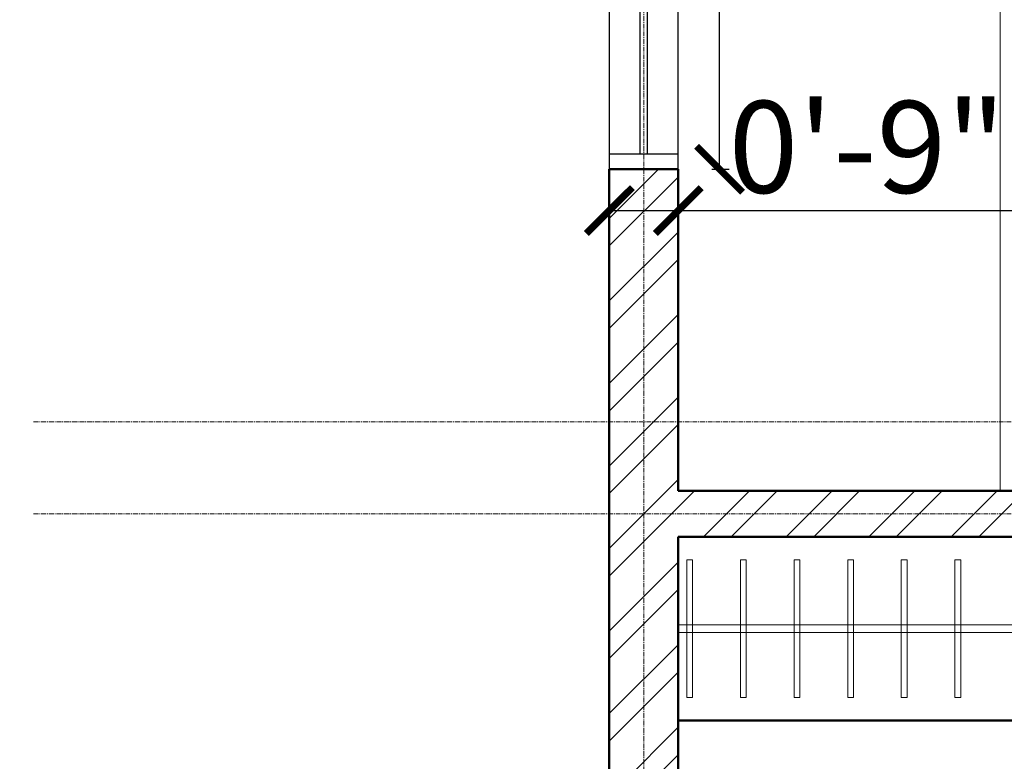
# Model space of a CAD drawing. Units: inches. Extents: x 261 to 2725, y 291 to 1454.
# Tile 19 of 35: x 1166 to 1295, y 644 to 741. Entities that reach past the tile are written whole.
import ezdxf

# ---------------------------------------------------------------- set-up
doc = ezdxf.new("R2010")
doc.units = ezdxf.units.IN
doc.linetypes.add('CENTER', pattern=[2, 1.25, -0.25, 0.25, -0.25])
for name, color, linetype, lineweight in [('A-ANNO-DIMS', 136, 'Continuous', 18), ('A-FLOR-FIXT', 145, 'Continuous', 18), ('A-FURN', 30, 'Continuous', 18), ('A-GLAZ', 150, 'Continuous', 25), ('A-GRID', 251, 'CENTER', 13), ('A-WALL', 222, 'Continuous', 50), ('A-WALL-PATT', 243, 'Continuous', 13)]:
    doc.layers.add(name, color=color, linetype=linetype, lineweight=lineweight)
doc.styles.get("Standard").update_dxf_attribs({"font": 'arial.ttf'})
doc.dimstyles.new('ISO-25', dxfattribs={"dimtxt": 12, "dimasz": 6, "dimexe": 1.25, "dimexo": 0.625, "dimtad": 1, "dimdec": 0, "dimlunit": 3, "dimtxsty": 'Standard', "dimblk": 'ARCHTICK', "dimcen": 2.5, "dimadec": 0, "dimazin": 0, "dimtfac": 1, "dimtdec": 0, "dimtmove": 0, "dimatfit": 3, "dimfxl": 1, "dimfxlon": 1, "dimarcsym": 0})

# ---------------------------------------------------------------- blocks, each defined once
blk = doc.blocks.new('WIN-36')
for p, q in [((1252.08, 755.47), (1243.08, 755.47)), ((1247.08, 755.47), (1247.08, 723.47)), ((1248.08, 723.47), (1248.08, 755.47)), ((1243.08, 723.47), (1252.08, 723.47))]:
    blk.add_line(p, q)
blk.add_lwpolyline([(1252.08, 721.47), (1252.08, 757.47), (1243.08, 757.47), (1243.08, 721.47)], close=True)
blk = doc.blocks.new('_ArchTick')
at = {"color": 0, "linetype": 'ByBlock', "const_width": 0.15}
blk.add_lwpolyline([(-0.5, -0.5), (0.5, 0.5)], dxfattribs=at)
blk = doc.blocks.new('*D59')
at = {"layer": 'A-ANNO-DIMS', "color": 0, "lineweight": -2, "ltscale": 0.07, "transparency": 16777216}
for p, q in [((1257.48, 757.47), (1257.48, 946.37)), ((1256.48, 757.47), (1258.73, 757.47)), ((1257.48, 721.47), (1257.48, 757.47)), ((1256.48, 721.47), (1258.73, 721.47))]:
    blk.add_line(p, q, dxfattribs=at)
at = {"layer": 'Defpoints', "color": 0, "ltscale": 0.07, "transparency": 16777216}
for p in [(1252.08, 757.47), (1257.48, 757.47), (1252.08, 721.47)]:
    blk.add_point(p, dxfattribs=at)
at = {"layer": 'A-ANNO-DIMS', "color": 0, "lineweight": -2, "ltscale": 0.07, "transparency": 16777216, "xscale": 6, "yscale": 6, "zscale": 6}
for p, rotation in [((1257.48, 757.47), 90), ((1257.48, 721.47), 270)]:
    blk.add_blockref('_ArchTick', p, dxfattribs=dict(at, rotation=rotation))
at = {"layer": 'A-ANNO-DIMS', "color": 0, "ltscale": 0.07, "transparency": 16777216, "insert": (1250.64, 854.92), "char_height": 12, "attachment_point": 5, "rotation": 90}
blk.add_mtext('WINDOW W3 3\'-0" TYP.', dxfattribs=at)
blk = doc.blocks.new('*D60')
at = {"layer": 'A-ANNO-DIMS', "color": 0, "lineweight": -2, "ltscale": 0.07, "transparency": 16777216}
for p, q in [((1243.08, 717.07), (1243.08, 714.82)), ((1243.08, 716.07), (1252.08, 716.07)), ((1252.08, 717.07), (1252.08, 714.82)), ((1252.08, 716.07), (1332.48, 716.07))]:
    blk.add_line(p, q, dxfattribs=at)
at = {"layer": 'Defpoints', "color": 0, "ltscale": 0.07, "transparency": 16777216}
for p in [(1243.08, 721.47), (1252.08, 721.47), (1252.08, 716.07)]:
    blk.add_point(p, dxfattribs=at)
at = {"layer": 'A-ANNO-DIMS', "color": 0, "lineweight": -2, "ltscale": 0.07, "transparency": 16777216, "xscale": 6, "yscale": 6, "zscale": 6, "rotation": 180}
blk.add_blockref('_ArchTick', (1243.08, 716.07), dxfattribs=at)
at = {"layer": 'A-ANNO-DIMS', "color": 0, "lineweight": -2, "ltscale": 0.07, "transparency": 16777216, "xscale": 6, "yscale": 6, "zscale": 6}
blk.add_blockref('_ArchTick', (1252.08, 716.07), dxfattribs=at)
at = {"layer": 'A-ANNO-DIMS', "color": 0, "ltscale": 0.07, "transparency": 16777216, "insert": (1295.28, 722.82), "char_height": 12, "attachment_point": 5}
blk.add_mtext('0\'-9" TYP.', dxfattribs=at)
blk = doc.blocks.new('*D82')
at = {"layer": 'A-ANNO-DIMS', "color": 0, "lineweight": -2, "ltscale": 0.07, "transparency": 16777216}
for p, q in [((2600.96, 679.47), (2603.21, 679.47)), ((2601.96, 517.47), (2601.96, 679.47)), ((2600.96, 517.47), (2603.21, 517.47))]:
    blk.add_line(p, q, dxfattribs=at)
at = {"layer": 'Defpoints', "color": 0, "ltscale": 0.07, "transparency": 16777216}
for p in [(946.45, 679.47), (2601.96, 679.47), (946.45, 517.47)]:
    blk.add_point(p, dxfattribs=at)
at = {"layer": 'A-ANNO-DIMS', "color": 0, "lineweight": -2, "ltscale": 0.07, "transparency": 16777216, "xscale": 6, "yscale": 6, "zscale": 6}
for p, rotation in [((2601.96, 679.47), 90), ((2601.96, 517.47), 270)]:
    blk.add_blockref('_ArchTick', p, dxfattribs=dict(at, rotation=rotation))
at = {"layer": 'A-ANNO-DIMS', "color": 0, "ltscale": 0.07, "transparency": 16777216, "insert": (2595.2, 598.47), "char_height": 12, "attachment_point": 5, "rotation": 90}
blk.add_mtext('13\'-6"', dxfattribs=at)
blk = doc.blocks.new('*D83')
at = {"layer": 'A-ANNO-DIMS', "color": 0, "lineweight": -2, "ltscale": 0.07, "transparency": 16777216}
for p, q in [((2600.96, 799.47), (2603.21, 799.47)), ((2601.96, 679.47), (2601.96, 799.47)), ((2600.96, 679.47), (2603.21, 679.47))]:
    blk.add_line(p, q, dxfattribs=at)
at = {"layer": 'Defpoints', "color": 0, "ltscale": 0.07, "transparency": 16777216}
for p in [(946.45, 799.47), (2601.96, 799.47), (946.45, 679.47)]:
    blk.add_point(p, dxfattribs=at)
at = {"layer": 'A-ANNO-DIMS', "color": 0, "lineweight": -2, "ltscale": 0.07, "transparency": 16777216, "xscale": 6, "yscale": 6, "zscale": 6}
for p, rotation in [((2601.96, 799.47), 90), ((2601.96, 679.47), 270)]:
    blk.add_blockref('_ArchTick', p, dxfattribs=dict(at, rotation=rotation))
at = {"layer": 'A-ANNO-DIMS', "color": 0, "ltscale": 0.07, "transparency": 16777216, "insert": (2595.21, 739.47), "char_height": 12, "attachment_point": 5, "rotation": 90}
blk.add_mtext('10\'-0"', dxfattribs=at)
blk = doc.blocks.new('*D103')
at = {"layer": 'A-ANNO-DIMS', "color": 0, "lineweight": -2, "ltscale": 0.07, "transparency": 16777216}
for p, q in [((287.06, 1231.47), (284.81, 1231.47)), ((286.06, 439.47), (286.06, 1231.47)), ((287.06, 439.47), (284.81, 439.47))]:
    blk.add_line(p, q, dxfattribs=at)
at = {"layer": 'Defpoints', "color": 0, "ltscale": 0.07, "transparency": 16777216}
for p in [(286.06, 1231.47), (1243.08, 1231.47), (1243.08, 439.47)]:
    blk.add_point(p, dxfattribs=at)
at = {"layer": 'A-ANNO-DIMS', "color": 0, "lineweight": -2, "ltscale": 0.07, "transparency": 16777216, "xscale": 6, "yscale": 6, "zscale": 6}
for p, rotation in [((286.06, 1231.47), 90), ((286.06, 439.47), 270)]:
    blk.add_blockref('_ArchTick', p, dxfattribs=dict(at, rotation=rotation))
at = {"layer": 'A-ANNO-DIMS', "color": 0, "ltscale": 0.07, "transparency": 16777216, "insert": (279.3, 835.47), "char_height": 12, "attachment_point": 5, "rotation": 90}
blk.add_mtext('66\'-0"', dxfattribs=at)
blk = doc.blocks.new('*D107')
at = {"layer": 'A-ANNO-DIMS', "color": 0, "lineweight": -2, "ltscale": 0.07, "transparency": 16777216}
for p, q in [((287.06, 673.47), (284.81, 673.47)), ((286.06, 496.47), (286.06, 673.47)), ((287.06, 496.47), (284.81, 496.47))]:
    blk.add_line(p, q, dxfattribs=at)
at = {"layer": 'Defpoints', "color": 0, "ltscale": 0.07, "transparency": 16777216}
for p in [(286.06, 673.47), (1252.08, 673.47), (1252.08, 496.47)]:
    blk.add_point(p, dxfattribs=at)
at = {"layer": 'A-ANNO-DIMS', "color": 0, "lineweight": -2, "ltscale": 0.07, "transparency": 16777216, "xscale": 6, "yscale": 6, "zscale": 6}
for p, rotation in [((286.06, 673.47), 90), ((286.06, 496.47), 270)]:
    blk.add_blockref('_ArchTick', p, dxfattribs=dict(at, rotation=rotation))
at = {"layer": 'A-ANNO-DIMS', "color": 0, "ltscale": 0.07, "transparency": 16777216, "insert": (279.3, 584.97), "char_height": 12, "attachment_point": 5, "rotation": 90}
blk.add_mtext('14\'-9"', dxfattribs=at)
blk = doc.blocks.new('*D108')
at = {"layer": 'A-ANNO-DIMS', "color": 0, "lineweight": -2, "ltscale": 0.07, "transparency": 16777216}
for p, q in [((287.06, 799.47), (284.81, 799.47)), ((286.06, 673.47), (286.06, 799.47)), ((287.06, 673.47), (284.81, 673.47))]:
    blk.add_line(p, q, dxfattribs=at)
at = {"layer": 'Defpoints', "color": 0, "ltscale": 0.07, "transparency": 16777216}
for p in [(286.06, 799.47), (1252.08, 799.47), (1252.08, 673.47)]:
    blk.add_point(p, dxfattribs=at)
at = {"layer": 'A-ANNO-DIMS', "color": 0, "lineweight": -2, "ltscale": 0.07, "transparency": 16777216, "xscale": 6, "yscale": 6, "zscale": 6}
for p, rotation in [((286.06, 799.47), 90), ((286.06, 673.47), 270)]:
    blk.add_blockref('_ArchTick', p, dxfattribs=dict(at, rotation=rotation))
at = {"layer": 'A-ANNO-DIMS', "color": 0, "ltscale": 0.07, "transparency": 16777216, "insert": (279.3, 736.47), "char_height": 12, "attachment_point": 5, "rotation": 90}
blk.add_mtext('10\'-6"', dxfattribs=at)
blk = doc.blocks.new('*D123')
at = {"layer": 'A-ANNO-DIMS', "color": 0, "lineweight": -2, "ltscale": 0.07, "transparency": 16777216}
for p, q in [((287.06, 1054.85), (284.81, 1054.85)), ((286.06, 439.47), (286.06, 1054.85)), ((287.06, 439.47), (284.81, 439.47))]:
    blk.add_line(p, q, dxfattribs=at)
at = {"layer": 'Defpoints', "color": 0, "ltscale": 0.07, "transparency": 16777216}
for p in [(286.06, 1054.85), (2007.71, 1054.85), (2007.71, 439.47)]:
    blk.add_point(p, dxfattribs=at)
at = {"layer": 'A-ANNO-DIMS', "color": 0, "lineweight": -2, "ltscale": 0.07, "transparency": 16777216, "xscale": 6, "yscale": 6, "zscale": 6}
for p, rotation in [((286.06, 1054.85), 90), ((286.06, 439.47), 270)]:
    blk.add_blockref('_ArchTick', p, dxfattribs=dict(at, rotation=rotation))
at = {"layer": 'A-ANNO-DIMS', "color": 0, "ltscale": 0.07, "transparency": 16777216, "insert": (279.22, 747.16), "char_height": 12, "attachment_point": 5, "rotation": 90}
blk.add_mtext('51\'-3 1/2"', dxfattribs=at)

msp = doc.modelspace()

# ---------------------------------------------------------------- hatches: boundary and pattern name
at = {"layer": 'A-WALL-PATT'}
h = msp.add_hatch(dxfattribs=at)
h.set_pattern_fill('ANSI32', color=256, scale=0.8)
h.paths.add_polyline_path([(478.45, 685.47), (580.45, 685.47), (580.45, 691.47), (577.45, 691.47), (577.45, 694.47), (571.45, 694.47), (571.45, 691.47), (478.45, 691.47), (478.45, 721.47), (469.45, 721.47), (469.45, 508.47), (538.45, 508.47), (538.45, 517.47), (478.45, 517.47)])
h.paths.add_polyline_path([(694.45, 517.47), (676.45, 517.47), (676.45, 646.47), (670.45, 646.47), (670.45, 517.47), (610.45, 517.47), (610.45, 508.47), (694.45, 508.47)])
h.paths.add_polyline_path([(676.45, 784.47), (478.45, 784.47), (478.45, 844.47), (469.45, 844.47), (469.45, 745.47), (478.45, 745.47), (478.45, 775.47), (571.45, 775.47), (571.45, 724.47), (577.45, 724.47), (577.45, 775.47), (670.45, 775.47), (670.45, 691.47), (610.45, 691.47), (610.45, 685.47), (670.45, 685.47), (670.45, 682.47), (676.45, 682.47)])
h.paths.add_polyline_path([(955.45, 880.47), (946.45, 880.47), (946.45, 808.47), (778.45, 808.47), (778.45, 799.47), (946.45, 799.47), (946.45, 517.47), (898.45, 517.47), (898.45, 508.47), (955.45, 508.47)])
h.paths.add_polyline_path([(778.45, 598.47), (772.45, 598.47), (772.45, 517.47), (754.45, 517.47), (754.45, 508.47), (826.45, 508.47), (826.45, 517.47), (778.45, 517.47)])
h.paths.add_polyline_path([(955.45, 1090.47), (946.45, 1090.47), (946.45, 1030.47), (817.45, 1030.47), (817.45, 1024.47), (946.45, 1024.47), (946.45, 952.47), (955.45, 952.47)])
h.paths.add_polyline_path([(955.45, 1231.47), (730.45, 1231.47), (730.45, 1222.47), (772.45, 1222.47), (772.45, 1096.47), (766.45, 1096.47), (766.45, 1090.47), (772.45, 1090.47), (772.45, 1006.47), (712.45, 1006.47), (712.45, 1000.47), (778.45, 1000.47), (778.45, 1024.47), (781.45, 1024.47), (781.45, 1030.47), (778.45, 1030.47), (778.45, 1222.47), (946.45, 1222.47), (946.45, 1162.47), (955.45, 1162.47)])
h.paths.add_polyline_path([(694.45, 1231.47), (619.45, 1231.47), (619.45, 1222.47), (646.45, 1222.47), (646.45, 1039.47), (652.45, 1039.47), (652.45, 1090.47), (736.45, 1090.47), (736.45, 1096.47), (652.45, 1096.47), (652.45, 1222.47), (694.45, 1222.47)])
h.paths.add_polyline_path([(571.45, 1231.47), (469.45, 1231.47), (469.45, 1099.47), (478.45, 1099.47), (478.45, 1144.47), (544.45, 1144.47), (544.45, 1153.47), (538.45, 1153.47), (538.45, 1150.47), (478.45, 1150.47), (478.45, 1222.47), (538.45, 1222.47), (538.45, 1183.47), (544.45, 1183.47), (544.45, 1222.47), (571.45, 1222.47)])
h.paths.add_polyline_path([(538.45, 1006.47), (478.45, 1006.47), (478.45, 1051.47), (469.45, 1051.47), (469.45, 940.47), (478.45, 940.47), (478.45, 1000.47), (538.45, 1000.47)])
h.paths.add_polyline_path([(652.45, 1006.47), (652.45, 1009.47), (646.45, 1009.47), (646.45, 1006.47), (586.45, 1006.47), (586.45, 1000.47), (652.45, 1000.47)])
h.paths.add_polyline_path([(1288.08, 973.47), (1243.08, 973.47), (1243.08, 920.97), (1252.08, 920.97), (1252.08, 964.47), (1288.08, 964.47)], flags=17)
h.paths.add_polyline_path([(1402.08, 805.47), (1252.08, 805.47), (1252.08, 848.97), (1243.08, 848.97), (1243.08, 757.47), (1252.08, 757.47), (1252.08, 799.47), (1294.08, 799.47), (1372.08, 799.47), (1372.08, 779.47), (1372.08, 715.47), (1378.08, 715.47), (1378.08, 799.47), (1402.08, 799.47)])
h.paths.add_polyline_path([(1252.08, 721.47), (1243.08, 721.47), (1243.08, 439.47), (1729.08, 439.47), (1729.08, 709.47), (1720.08, 709.47), (1720.08, 679.47), (1582.08, 679.47), (1582.08, 670.47), (1588.08, 670.47), (1588.08, 673.47), (1720.08, 673.47), (1720.08, 559.47), (1690.08, 559.47), (1690.08, 550.47), (1720.08, 550.47), (1720.08, 448.47), (1252.08, 448.47), (1252.08, 496.47), (1312.08, 496.47), (1312.08, 505.47), (1252.08, 505.47), (1252.08, 673.47), (1405.08, 673.47), (1405.08, 679.47), (1378.08, 679.47), (1378.08, 685.47), (1372.08, 685.47), (1372.08, 679.47), (1252.08, 679.47)])
h.paths.add_polyline_path([(1450.08, 550.47), (1480.08, 550.47), (1480.08, 559.47), (1450.08, 559.47), (1450.08, 679.47), (1441.08, 679.47), (1441.08, 673.47), (1444.08, 673.47), (1444.08, 505.47), (1384.08, 505.47), (1384.08, 496.47), (1450.08, 496.47)], flags=17)
h.paths.add_polyline_path([(1618.08, 559.47), (1588.08, 559.47), (1588.08, 634.47), (1582.08, 634.47), (1582.08, 559.47), (1552.08, 559.47), (1552.08, 550.47), (1618.08, 550.47)], flags=17)
h.paths.add_polyline_path([(1564.08, 964.47), (1630.08, 964.47), (1630.08, 973.47), (1477.08, 973.47), (1477.08, 964.47), (1558.08, 964.47), (1558.08, 926.22), (1558.08, 887.97), (1486.08, 887.97), (1486.08, 881.97), (1558.08, 881.97), (1558.08, 805.47), (1450.08, 805.47), (1450.08, 845.97), (1444.08, 845.97), (1444.08, 805.47), (1438.08, 805.47), (1438.08, 799.47), (1564.08, 799.47)], flags=17)
h.paths.add_polyline_path([(1453.08, 973.47), (1408.08, 973.47), (1408.08, 964.47), (1444.08, 964.47), (1444.08, 881.97), (1450.08, 881.97), (1456.08, 881.97), (1456.08, 887.97), (1450.08, 887.97), (1450.08, 964.47), (1453.08, 964.47)], flags=17)
h.paths.add_polyline_path([(1729.08, 1231.47), (1243.08, 1231.47), (1243.08, 1167.47), (1252.08, 1167.47), (1252.08, 1222.47), (1441.08, 1222.47), (1441.08, 1045.47), (1648.08, 1045.47), (1648.08, 1051.47), (1450.08, 1051.47), (1450.08, 1074.47), (1450.08, 1222.47), (1472.08, 1222.47), (1720.08, 1222.47), (1720.08, 1051.47), (1708.08, 1051.47), (1708.08, 1045.47), (1720.08, 1045.47), (1720.08, 973.47), (1702.08, 973.47), (1702.08, 964.47), (1720.08, 964.47), (1720.08, 769.47), (1729.08, 769.47)])
h.paths.add_polyline_path([(2493.71, 1054.85), (2007.71, 1054.85), (2007.71, 439.47), (2214.67, 439.47), (2214.67, 496.47), (2493.71, 496.47)])
h.paths.add_polyline_path([(2016.71, 1045.85), (2304.71, 1045.85), (2304.71, 841.47), (2310.71, 841.47), (2310.71, 1045.85), (2484.71, 1045.85), (2484.71, 805.47), (2310.71, 805.47), (2310.71, 811.47), (2304.71, 811.47), (2304.71, 799.47), (2484.71, 799.47), (2484.71, 679.47), (2304.71, 679.47), (2304.71, 673.47), (2484.71, 673.47), (2484.71, 505.47), (2208.67, 505.47), (2208.67, 448.47), (2016.71, 448.47), (2016.71, 799.47), (2304.71, 799.47), (2304.71, 805.47), (2016.71, 805.47)], flags=16)

# ---------------------------------------------------------------- linework, layer by layer
at = {"layer": 'A-FLOR-FIXT'}
msp.add_lwpolyline([(1252.08, 679.47), (1294.08, 679.47), (1294.08, 799.47), (1252.08, 799.47)], close=True, dxfattribs=at)
at = {"layer": 'A-FURN'}
for p, q in [((1348.08, 661.97), (1252.08, 661.97)), ((1348.08, 660.97), (1252.08, 660.97))]:
    msp.add_line(p, q, dxfattribs=at)
for points in [[(1253.2, 670.47), (1253.2, 652.47), (1253.95, 652.47), (1253.95, 670.47)], [(1260.2, 670.47), (1260.2, 652.47), (1260.95, 652.47), (1260.95, 670.47)], [(1267.2, 670.47), (1267.2, 652.47), (1267.95, 652.47), (1267.95, 670.47)], [(1274.2, 670.47), (1274.2, 652.47), (1274.95, 652.47), (1274.95, 670.47)], [(1281.2, 670.47), (1281.2, 652.47), (1281.95, 652.47), (1281.95, 670.47)], [(1288.2, 670.47), (1288.2, 652.47), (1288.95, 652.47), (1288.95, 670.47)]]:
    msp.add_lwpolyline(points, close=True, dxfattribs=at)
at = {"layer": 'A-GRID', "ltscale": 0.5}
for p, q in [((1247.58, 1330.47), (1247.58, 416.47)), ((1167.93, 688.47), (1791.93, 688.47)), ((1167.93, 676.47), (1791.93, 676.47))]:
    msp.add_line(p, q, dxfattribs=at)
at = {"layer": 'A-WALL'}
for p, q in [((1243.08, 439.47), (1243.08, 721.47)), ((1252.08, 721.47), (1243.08, 721.47)), ((1252.08, 679.47), (1252.08, 721.47)), ((1252.08, 679.47), (1372.08, 679.47)), ((1252.08, 673.47), (1405.08, 673.47)), ((1252.08, 505.47), (1252.08, 673.47)), ((1252.08, 649.47), (1348.08, 649.47))]:
    msp.add_line(p, q, dxfattribs=at)

# ---------------------------------------------------------------- block references
at = {"layer": 'A-GLAZ'}
msp.add_blockref('WIN-36', (0, 0), dxfattribs=at)

# ---------------------------------------------------------------- dimensions: what is measured, and where the dimension line sits
at = {"layer": 'A-ANNO-DIMS', "ltscale": 0.07}
for base, p1, p2, picture, middle in [((286.06, 1231.47), (1243.08, 439.47), (1243.08, 1231.47), '*D103', (279.3, 835.47)), ((286.06, 1054.85), (2007.71, 439.47), (2007.71, 1054.85), '*D123', (279.22, 747.16)), ((286.06, 799.47), (1252.08, 673.47), (1252.08, 799.47), '*D108', (279.3, 736.47)), ((2601.96, 799.47), (946.45, 679.47), (946.45, 799.47), '*D83', (2595.21, 739.47)), ((2601.96, 679.47), (946.45, 517.47), (946.45, 679.47), '*D82', (2595.2, 598.47)), ((286.06, 673.47), (1252.08, 496.47), (1252.08, 673.47), '*D107', (279.3, 584.97))]:
    dim = msp.add_linear_dim(base=base, p1=p1, p2=p2, angle=90, dimstyle='ISO-25', override={"dimdec": 1, "dimlfac": 1, "dimrnd": 0, "dimzin": 1, "dimdsep": 46, "dimlunit": 4, "dimfrac": 2}, dxfattribs=at)
    dim.commit()
    dim.dimension.update_dxf_attribs({"geometry": picture, "text_midpoint": middle})
dim = msp.add_linear_dim(base=(1257.48, 757.47), p1=(1252.08, 721.47), p2=(1252.08, 757.47), angle=90, text='WINDOW W3 <> TYP.', dimstyle='ISO-25', override={"dimdec": 1, "dimrnd": 0, "dimzin": 1, "dimlunit": 4, "dimfrac": 2}, dxfattribs=at)
dim.commit()
dim.dimension.update_dxf_attribs({"geometry": '*D59', "text_midpoint": (1250.64, 854.92)})
dim = msp.add_linear_dim(base=(1252.08, 716.07), p1=(1243.08, 721.47), p2=(1252.08, 721.47), text='<> TYP.', dimstyle='ISO-25', override={"dimdec": 1, "dimrnd": 0, "dimzin": 1, "dimlunit": 4, "dimfrac": 2}, dxfattribs=at)
dim.commit()
dim.dimension.update_dxf_attribs({"geometry": '*D60', "text_midpoint": (1295.28, 722.82)})

doc.saveas('drawing.dxf')
